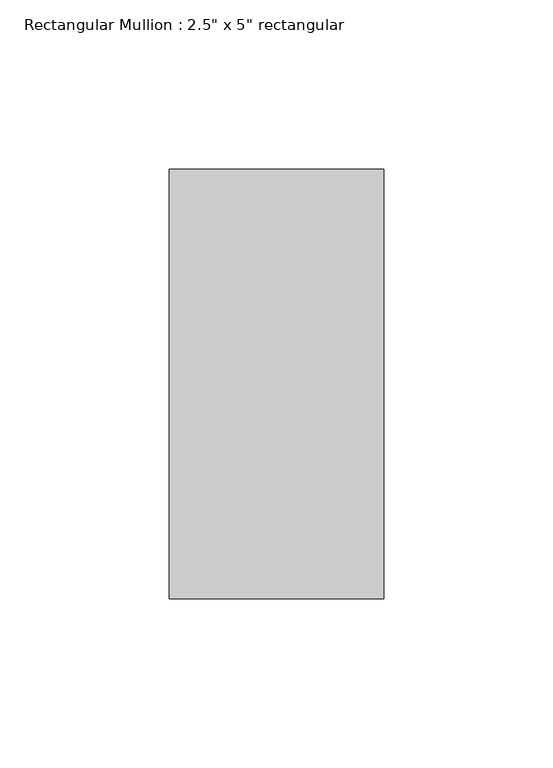
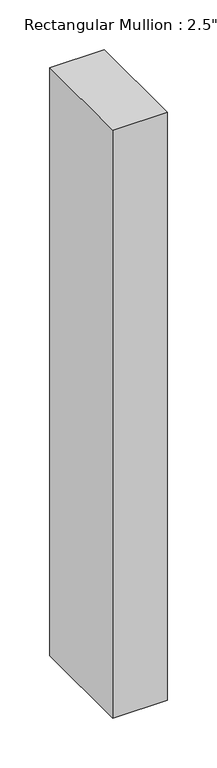
"""IFC4 building model written with IfcOpenShell, lengths in millimetres: member geometry."""

from ifc_helpers import new_model, si_unit, frame, origin, place, context, project, spatial, polyline, outline, extrude, source, transform, mapped, element, save


def member_0c11e56c(model_context):
    return source(origin(), model_context, "Body", "SweptSolid", [
        extrude(outline(polyline([(31.75, 63.5), (31.75, -63.5), (-31.75, -63.5), (-31.75, 63.5), (31.75, 63.5)])), frame((0.0, 0.0, -724.0034475), z_axis=(0.0, 0.0, 1.0), x_axis=(1.0, 0.0, 0.0)), (0.0, 0.0, 1.0), 724.0034475),
    ])


if __name__ == "__main__":
    model = new_model("IFC4")
    model_context = context("Model", 3, world=origin())
    ifc_project = project(units=[si_unit("LENGTHUNIT", "METRE", prefix="MILLI")], contexts=[model_context])
    site = spatial("IfcSite", under=ifc_project)
    building = spatial("IfcBuilding", under=site)
    placement = place(None, origin())
    member_shape = member_0c11e56c(model_context)
    element("IfcMember", 1, ObjectType="Rectangular Mullion : 2.5\" x 5\" rectangular", at=placement, inside=building, context=model_context, shape_type="MappedRepresentation", body=[
        mapped(member_shape, transform((0.0, 0.0, 0.0), x_axis=(1.0, 0.0, 0.0), y_axis=(0.0, 1.0, 0.0), z_axis=(0.0, 0.0, 1.0))),
    ])
    save(model, "model.ifc")

# Revit data of these elements
# Type "Rectangular Mullion : 2.5\" x 5\" rectangular"
#   built-in parameter 1007304 = 0.416667 (stored number, unit not read)
#   built-in parameter 1007301 = 0.104167 (stored number, unit not read)
#   built-in parameter 1007300 = 0.104167 (stored number, unit not read)
# Element 1 (IfcMember, "Rectangular Mullion : 2.5\" x 5\" rectangular")
#   Materials on its faces: "Aluminum"
# Materials
#   "Aluminum": class "Metal", colour RGB 247 247 247, transparency 0, Description = "Aluminum 6061", Cost = 0
